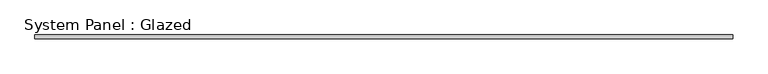
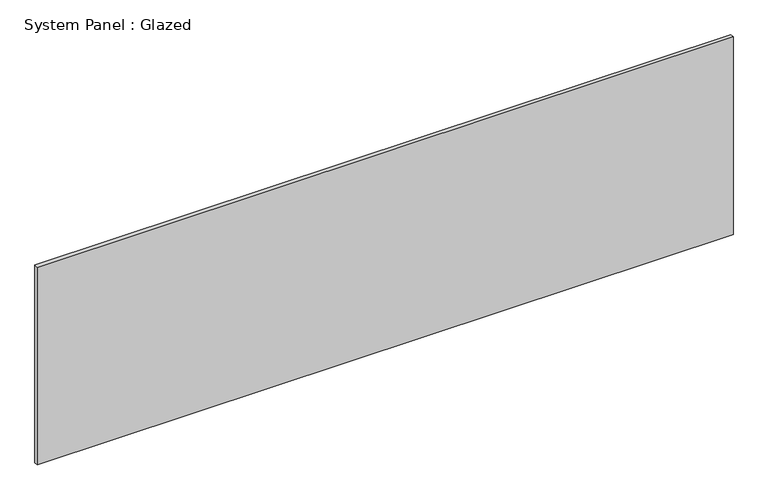
"""IFC4 building model written with IfcOpenShell, lengths in millimetres: plate geometry, System Panel : Glazed."""

from ifc_helpers import new_model, si_unit, origin, origin_with_axes, place, context, project, spatial, polyline, outline, extrude, source, transform, mapped, element, save


def system_panel_glazed_ba9ccfd0(model_context):
    return source(origin(), model_context, "Body", "SweptSolid", [
        extrude(outline(polyline([(2428.875, 19.05), (-2428.875, 19.05), (-2428.875, 44.45), (2428.875, 44.45), (2428.875, 19.05)])), origin_with_axes(), (0.0, 0.0, 1.0), 1460.5),
    ])


if __name__ == "__main__":
    model = new_model("IFC4")
    model_context = context("Model", 3, world=origin())
    ifc_project = project(units=[si_unit("LENGTHUNIT", "METRE", prefix="MILLI")], contexts=[model_context])
    site = spatial("IfcSite", under=ifc_project)
    building = spatial("IfcBuilding", under=site)
    placement = place(None, origin())
    system_panel_glazed_shape = system_panel_glazed_ba9ccfd0(model_context)
    element("IfcPlate", 1, ObjectType="System Panel : Glazed", at=placement, inside=building, context=model_context, shape_type="MappedRepresentation", body=[
        mapped(system_panel_glazed_shape, transform((0.0, 0.0, 0.0), x_axis=(1.0, 0.0, 0.0), y_axis=(0.0, 1.0, 0.0), z_axis=(0.0, 0.0, 1.0))),
    ])
    save(model, "model.ifc")

# Revit data of these elements
# Type "System Panel : Glazed"
#   Construction Type Id = "GSP4R"
#   Analytic Construction = "1/8 in Pilkington single glazing"
#   Visual Light Transmittance = 0.9
#   Solar Heat Gain Coefficient = 0.86
#   Heat Transfer Coefficient (U) = 1.18115 BTU/(h·ft²·°F)
# Element 1 (IfcPlate, "System Panel : Glazed")
#   Materials on its faces: "Glass"
# Materials
#   "Glass": class "Glass", colour RGB 0 128 192, transparency 0.75, Description = "Soda Lime Glass", Cost = 0
